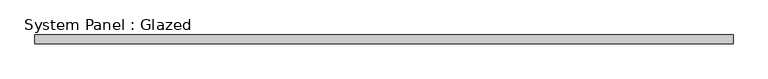
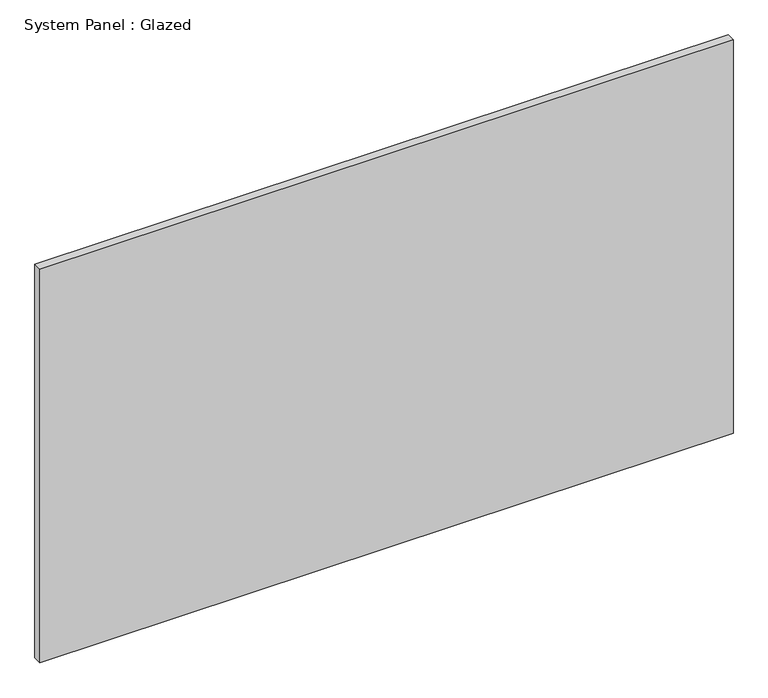
"""IFC4 building model written with IfcOpenShell, lengths in millimetres: plate geometry, System Panel : Glazed."""

from ifc_helpers import new_model, si_unit, origin, origin_with_axes, place, context, project, spatial, polyline, outline, extrude, source, transform, mapped, element, save


def system_panel_glazed_7481726a(model_context):
    return source(origin(), model_context, "Body", "SweptSolid", [
        extrude(outline(polyline([(1016.0, 19.05), (-1016.0, 19.05), (-1016.0, 44.45), (1016.0, 44.45), (1016.0, 19.05)])), origin_with_axes(), (0.0, 0.0, 1.0), 1219.2),
    ])


if __name__ == "__main__":
    model = new_model("IFC4")
    model_context = context("Model", 3, world=origin())
    ifc_project = project(units=[si_unit("LENGTHUNIT", "METRE", prefix="MILLI")], contexts=[model_context])
    site = spatial("IfcSite", under=ifc_project)
    building = spatial("IfcBuilding", under=site)
    placement = place(None, origin())
    system_panel_glazed_shape = system_panel_glazed_7481726a(model_context)
    element("IfcPlate", 1, ObjectType="System Panel : Glazed", at=placement, inside=building, context=model_context, shape_type="MappedRepresentation", body=[
        mapped(system_panel_glazed_shape, transform((0.0, 0.0, 0.0), x_axis=(1.0, 0.0, 0.0), y_axis=(0.0, 1.0, 0.0), z_axis=(0.0, 0.0, 1.0))),
    ])
    save(model, "model.ifc")

# Revit data of these elements
# Type "System Panel : Glazed"
#   Construction Type Id = "GSP4R"
#   Analytic Construction = "1/8 in Pilkington single glazing"
#   Visual Light Transmittance = 0.9
#   Solar Heat Gain Coefficient = 0.86
#   Heat Transfer Coefficient (U) = 1.18115 BTU/(h·ft²·°F)
# Element 1 (IfcPlate, "System Panel : Glazed")
#   Materials on its faces: "Glass"
# Materials
#   "Glass": class "Glass", colour RGB 0 128 192, transparency 0.75, Description = "Soda Lime Glass", Cost = 0
